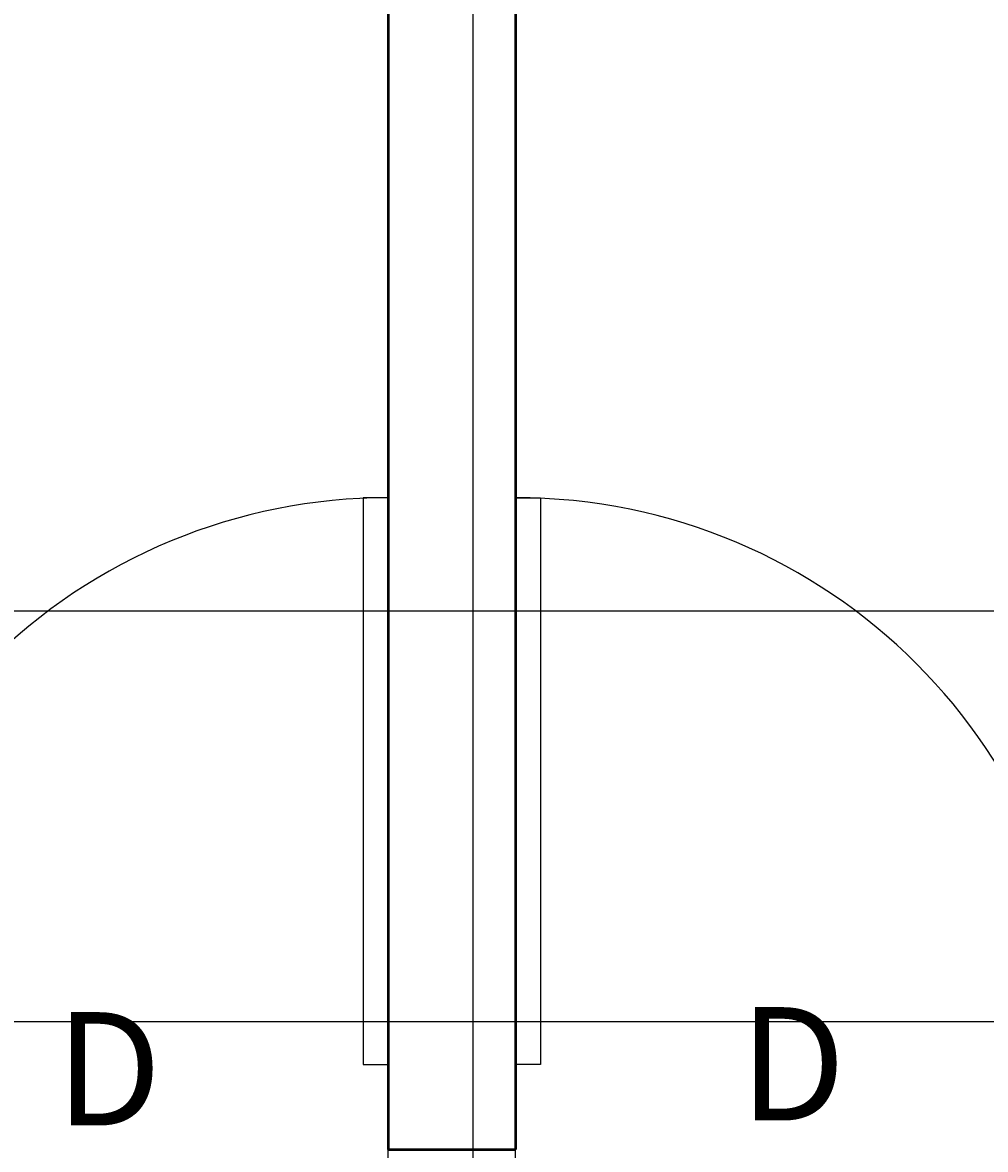
# Model space of a CAD drawing. Units: inches. Extents: x 37 to 824, y -700 to 234.
# Tile 68 of 77: x 264 to 332, y 75 to 155. Entities that reach past the tile are written whole.
import ezdxf

# ---------------------------------------------------------------- set-up
doc = ezdxf.new("R2010")
doc.units = ezdxf.units.IN
doc.header["$MEASUREMENT"] = 0
for name, color, linetype, lineweight in [('A-ANNO-DIMS', 2, 'Continuous', 18), ('A-ANNO-TEXT', 7, 'Continuous', 18), ('A-DOOR', 4, 'Continuous', 25), ('A-WALL', 2, 'Continuous', 50)]:
    doc.layers.add(name, color=color, linetype=linetype, lineweight=lineweight)
doc.styles.get("Standard").update_dxf_attribs({"font": 'arial.ttf'})
doc.dimstyles.get("Standard").update_dxf_attribs({"dimtxt": 0.18, "dimasz": 0.18, "dimexe": 0.18, "dimexo": 0.0625, "dimgap": 0.09, "dimtad": 0, "dimtih": 1, "dimtoh": 1, "dimdec": 1, "dimzin": 0, "dimdsep": 46, "dimlunit": 4, "dimtxsty": 'Standard', "dimcen": 0.09, "dimadec": 0, "dimazin": 0, "dimtfac": 1, "dimtdec": 1, "dimtofl": 0, "dimtmove": 0, "dimatfit": 3, "dimfxl": 1, "dimtolj": 1, "dimtzin": 0, "dimarcsym": 0})

# ---------------------------------------------------------------- blocks, each defined once
blk = doc.blocks.new('*U5')
for p, q in [((0, 0), (0, 6)), ((40, 0), (40, 6))]:
    blk.add_line(p, q)
blk.add_lwpolyline([(0, 0), (0, -40), (1.75, -40), (1.75, 0)], close=True)
blk.add_arc((0, 0), 40, 270, 0)
blk = doc.blocks.new('*U2')
for p, q in [((-40, 0), (-40, 6)), ((0, 0), (0, 6))]:
    blk.add_line(p, q)
blk.add_lwpolyline([(0, 0), (0, -40), (-1.75, -40), (-1.75, 0)], close=True)
blk.add_arc((0, 0), 40, 180, 270)
blk = doc.blocks.new('*D60')
at = {"layer": 'A-ANNO-DIMS', "color": 0, "lineweight": -2, "ltscale": 0.5, "transparency": 16777216}
for p, q in [((419.015, 113.09), (78.159, 113.09)), ((78.339, 112.91), (78.339, 98.772)), ((78.339, 84.27), (78.339, 98.409)), ((419.015, 84.09), (78.159, 84.09))]:
    blk.add_line(p, q, dxfattribs=at)
at = {"layer": 'A-ANNO-DIMS', "color": 0, "ltscale": 0.5, "transparency": 16777216}
for points in [[(78.309, 112.91), (78.369, 112.91), (78.339, 113.09)], [(78.309, 84.27), (78.369, 84.27), (78.339, 84.09)]]:
    blk.add_solid(points, dxfattribs=at)
at = {"layer": 'Defpoints', "color": 0, "ltscale": 0.5, "transparency": 16777216}
for p in [(78.339, 113.09), (419.077, 113.09), (419.077, 84.09)]:
    blk.add_point(p, dxfattribs=at)
at = {"layer": 'A-ANNO-DIMS', "color": 0, "ltscale": 0.5, "transparency": 16777216, "insert": (78.339, 98.59), "char_height": 0.18, "attachment_point": 5}
blk.add_mtext('\\A1;2\'-5"', dxfattribs=at)
blk = doc.blocks.new('*D73')
at = {"layer": 'A-ANNO-DIMS', "color": 0, "lineweight": -2, "ltscale": 0.5, "transparency": 16777216}
for p, q in [((250.19, 84.153), (250.19, 234.17)), ((250.37, 233.99), (269.804, 233.99)), ((289.897, 233.99), (270.463, 233.99)), ((290.077, 81.153), (290.077, 234.17))]:
    blk.add_line(p, q, dxfattribs=at)
at = {"layer": 'A-ANNO-DIMS', "color": 0, "ltscale": 0.5, "transparency": 16777216}
for points in [[(250.37, 234.02), (250.37, 233.96), (250.19, 233.99)], [(289.897, 234.02), (289.897, 233.96), (290.077, 233.99)]]:
    blk.add_solid(points, dxfattribs=at)
at = {"layer": 'Defpoints', "color": 0, "ltscale": 0.5, "transparency": 16777216}
for p in [(290.077, 233.99), (250.19, 84.09), (290.077, 81.09)]:
    blk.add_point(p, dxfattribs=at)
at = {"layer": 'A-ANNO-DIMS', "color": 0, "ltscale": 0.5, "transparency": 16777216, "insert": (270.133, 233.99), "char_height": 0.18, "attachment_point": 5}
blk.add_mtext('\\A1;3\'-4"', dxfattribs=at)
blk = doc.blocks.new('*D78')
at = {"layer": 'A-ANNO-DIMS', "color": 0, "lineweight": -2, "ltscale": 0.5, "transparency": 16777216}
for p, q in [((290.077, 15.153), (290.077, 234.17)), ((290.257, 233.99), (325.747, 233.99)), ((361.897, 233.99), (326.407, 233.99)), ((362.077, 15.153), (362.077, 234.17))]:
    blk.add_line(p, q, dxfattribs=at)
at = {"layer": 'A-ANNO-DIMS', "color": 0, "ltscale": 0.5, "transparency": 16777216}
for points in [[(290.257, 234.02), (290.257, 233.96), (290.077, 233.99)], [(361.897, 234.02), (361.897, 233.96), (362.077, 233.99)]]:
    blk.add_solid(points, dxfattribs=at)
at = {"layer": 'Defpoints', "color": 0, "ltscale": 0.5, "transparency": 16777216}
for p in [(362.077, 233.99), (290.077, 15.09), (362.077, 15.09)]:
    blk.add_point(p, dxfattribs=at)
at = {"layer": 'A-ANNO-DIMS', "color": 0, "ltscale": 0.5, "transparency": 16777216, "insert": (326.077, 233.99), "char_height": 0.18, "attachment_point": 5}
blk.add_mtext('\\A1;6\'-0"', dxfattribs=at)
blk = doc.blocks.new('*D82')
at = {"layer": 'A-ANNO-DIMS', "color": 0, "lineweight": -2, "ltscale": 0.5, "transparency": 16777216}
for p, q in [((299.077, -206.847), (299.077, 234.17)), ((299.257, 233.99), (328.202, 233.99)), ((357.952, 233.99), (329.008, 233.99)), ((358.132, -206.847), (358.132, 234.17))]:
    blk.add_line(p, q, dxfattribs=at)
at = {"layer": 'A-ANNO-DIMS', "color": 0, "ltscale": 0.5, "transparency": 16777216}
for points in [[(299.257, 234.02), (299.257, 233.96), (299.077, 233.99)], [(357.952, 234.02), (357.952, 233.96), (358.132, 233.99)]]:
    blk.add_solid(points, dxfattribs=at)
at = {"layer": 'Defpoints', "color": 0, "ltscale": 0.5, "transparency": 16777216}
for p in [(358.132, 233.99), (299.077, -206.91), (358.132, -206.91)]:
    blk.add_point(p, dxfattribs=at)
at = {"layer": 'A-ANNO-DIMS', "color": 0, "ltscale": 0.5, "transparency": 16777216, "insert": (328.605, 233.99), "char_height": 0.18, "attachment_point": 5}
blk.add_mtext('\\A1;4\'-11"', dxfattribs=at)
blk = doc.blocks.new('*D87')
at = {"layer": 'A-ANNO-DIMS', "color": 0, "lineweight": -2, "ltscale": 0.5, "transparency": 16777216}
for p, q in [((216.077, -356.847), (216.077, 234.17)), ((216.257, 233.99), (255.747, 233.99)), ((295.897, 233.99), (256.407, 233.99)), ((296.077, -356.847), (296.077, 234.17))]:
    blk.add_line(p, q, dxfattribs=at)
at = {"layer": 'A-ANNO-DIMS', "color": 0, "ltscale": 0.5, "transparency": 16777216}
for points in [[(216.257, 234.02), (216.257, 233.96), (216.077, 233.99)], [(295.897, 234.02), (295.897, 233.96), (296.077, 233.99)]]:
    blk.add_solid(points, dxfattribs=at)
at = {"layer": 'Defpoints', "color": 0, "ltscale": 0.5, "transparency": 16777216}
for p in [(296.077, 233.99), (216.077, -356.91), (296.077, -356.91)]:
    blk.add_point(p, dxfattribs=at)
at = {"layer": 'A-ANNO-DIMS', "color": 0, "ltscale": 0.5, "transparency": 16777216, "insert": (256.077, 233.99), "char_height": 0.18, "attachment_point": 5}
blk.add_mtext('\\A1;6\'-8"', dxfattribs=at)

msp = doc.modelspace()

# ---------------------------------------------------------------- linework, layer by layer
at = {"layer": 'A-WALL'}
for p, q in [((290.077, 182.09), (290.077, 75.09)), ((299.077, 182.09), (299.077, 75.09)), ((290.077, 75.09), (299.077, 75.09))]:
    msp.add_line(p, q, dxfattribs=at)

# ---------------------------------------------------------------- block references
at = {"layer": 'A-DOOR', "rotation": 180}
for name, p in [('*U5', (290.077, 81.09)), ('*U2', (299.077, 81.09))]:
    msp.add_blockref(name, p, dxfattribs=at)

# ---------------------------------------------------------------- texts
at = {"layer": 'A-ANNO-TEXT'}
for p in [(314.861, 77.136), (266.592, 76.782)]:
    msp.add_text('D', height=8, dxfattribs=at).set_placement(p)

# ---------------------------------------------------------------- dimensions: what is measured, and where the dimension line sits
at = {"layer": 'A-ANNO-DIMS', "ltscale": 0.5}
for base, p1, p2, picture, middle in [((296.077, 233.99), (216.077, -356.91), (296.077, -356.91), '*D87', (256.077, 233.99)), ((290.077, 233.99), (250.19, 84.09), (290.077, 81.09), '*D73', (270.133, 233.99)), ((362.077, 233.99), (290.077, 15.09), (362.077, 15.09), '*D78', (326.077, 233.99)), ((358.132, 233.99), (299.077, -206.91), (358.132, -206.91), '*D82', (328.605, 233.99))]:
    dim = msp.add_linear_dim(base=base, p1=p1, p2=p2, dimstyle='Standard', override={"dimdec": 1, "dimlfac": 1, "dimrnd": 0, "dimzin": 1, "dimdsep": 46, "dimlunit": 4, "dimfrac": 2}, dxfattribs=at)
    dim.commit()
    dim.dimension.update_dxf_attribs({"geometry": picture, "text_midpoint": middle})
dim = msp.add_linear_dim(base=(78.339, 113.09), p1=(419.077, 84.09), p2=(419.077, 113.09), angle=90, dimstyle='Standard', override={"dimdec": 1, "dimlfac": 1, "dimrnd": 0, "dimzin": 1, "dimdsep": 46, "dimlunit": 4, "dimfrac": 2}, dxfattribs=at)
dim.commit()
dim.dimension.update_dxf_attribs({"geometry": '*D60', "text_midpoint": (78.339, 98.59)})

doc.saveas('drawing.dxf')
